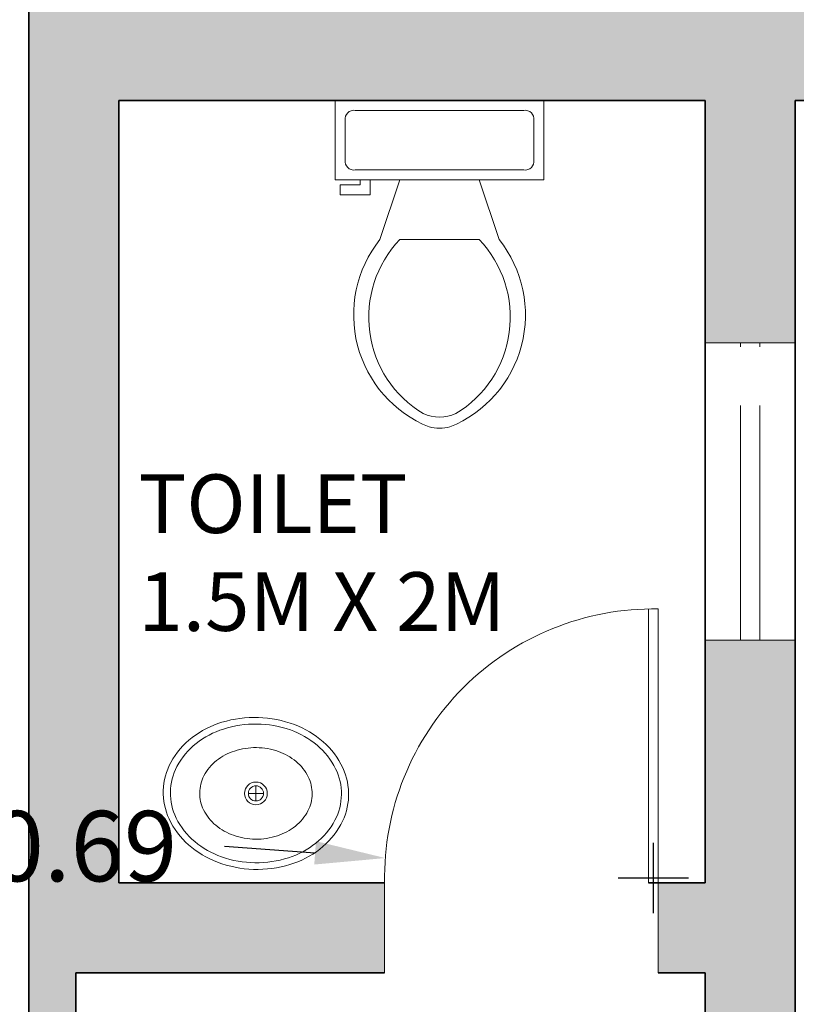
# Model space of a CAD drawing. Units: metres. Extents: x 4298.5 to 4325.2, y 2075 to 2095.8.
# Tile 28 of 35: x 4318.3 to 4320.3, y 2082.2 to 2084.8. Entities that reach past the tile are written whole.
import ezdxf

# ---------------------------------------------------------------- set-up
doc = ezdxf.new("R2010")
doc.units = ezdxf.units.M
doc.linetypes.add('ACAD_ISO02W100', pattern=[15, 12, -3])
for name, color, linetype, lineweight in [('A-ANNO-DIMS', 2, 'Continuous', 18), ('A-AREA-IDEN', 7, 'Continuous', 18), ('A-DOOR', 3, 'Continuous', 18), ('A-FLOR-FIXT', 15, 'Continuous', 18), ('A-GLAZ', 4, 'Continuous', 18), ('A-GLAZ-OVHD', 4, 'ACAD_ISO02W100', 13), ('A-WALL', 7, 'Continuous', 35), ('A-WALL-PATT', 252, 'Continuous', 13)]:
    doc.layers.add(name, color=color, linetype=linetype, lineweight=lineweight)
doc.styles.get("Standard").update_dxf_attribs({"font": 'arial.ttf'})
doc.dimstyles.get("Standard").update_dxf_attribs({"dimtxt": 0.18, "dimasz": 0.18, "dimexe": 0.18, "dimexo": 0.0625, "dimgap": 0.09, "dimtad": 0, "dimtih": 1, "dimtoh": 1, "dimdec": 4, "dimzin": 0, "dimdsep": 46, "dimtxsty": 'Standard', "dimcen": 0.09, "dimadec": 0, "dimazin": 0, "dimtfac": 1, "dimtdec": 4, "dimtofl": 0, "dimtmove": 0, "dimatfit": 3, "dimfxl": 1, "dimtolj": 1, "dimtzin": 0, "dimarcsym": 0})

# ---------------------------------------------------------------- blocks, each defined once
blk = doc.blocks.new('Toilet - top')
for p, q in [((9.5, -6), (9.5, -2)), ((-10, -8.5), (-8, -8.5)), ((-10, -9.5), (-10, -8.5)), ((-8, -8.5), (-8, -8)), ((-7, -8), (-7, -9.5)), ((-4, -8), (-6, -14)), ((4, -8), (6, -14)), ((-7, -9.5), (-10, -9.5)), ((4, -14), (-4, -14))]:
    blk.add_line(p, q)
blk.add_lwpolyline([(10.5, -8), (10.5, 0), (-10.5, 0), (-10.5, -8)], close=True)
for points in [[(8.5, -1), (-8.5, -1)], [(-9.5, -2), (-9.5, -6)], [(-8.5, -7), (8.5, -7)]]:
    blk.add_lwpolyline(points)
for centre, radius, start, end in [((-8.625, -1.875), 0.884, 81.8699, 188.1301), ((8.625, -1.875), 0.884, 351.8699, 98.1301), ((-8.625, -6.125), 0.884, 171.8699, 278.1301), ((8.625, -6.125), 0.884, 261.8699, 8.1301), ((3.52, -21.58), 12.169, 141.46911, 247.97143), ((4.2, -21.817), 11.329, 136.36773, 238.94682), ((-3.519, -21.58), 12.169, 292.02843, 38.53071), ((-4.2, -21.817), 11.329, 301.05301, 43.63209), ((0, -27.876), 4, 245.73182, 294.26817), ((0, -29), 4, 254.86053, 285.13947)]:
    blk.add_arc(centre, radius, start, end)
blk = doc.blocks.new('Sink - Oval top')
for p, q in [((-1, 0), (1, 0)), ((0, 1), (0, -1))]:
    blk.add_line(p, q)
for points in [[(-12.23, 0.39, 0.117634), (-11.46, -3.36, 0.104469), (-8.88, -6.8, 0.090016), (-5.08, -9.07, 0.08192), (-0.32, -10.02, 0.08192), (4.49, -9.38, 0.090016), (8.42, -7.36, 0.104469), (11.22, -4.09, 0.117634), (12.23, -0.39, 0.117634), (11.46, 3.36, 0.104469), (8.88, 6.8, 0.090016), (5.08, 9.07, 0.08192), (0.32, 10.02, 0.08192), (-4.49, 9.38, 0.090016), (-8.42, 7.36, 0.104469), (-11.22, 4.09, 0.117634)], [(-11.29, 0.16, 0.118622), (-10.52, -3.25, 0.104678), (-8.07, -6.36, 0.089562), (-4.54, -8.37, 0.081185), (-0.13, -9.15, 0.081185), (4.3, -8.49, 0.089562), (7.89, -6.58, 0.104678), (10.42, -3.55, 0.118622), (11.29, -0.16, 0.118622), (10.52, 3.25, 0.104678), (8.07, 6.36, 0.089562), (4.54, 8.37, 0.081185), (0.13, 9.15, 0.081185), (-4.3, 8.49, 0.089562), (-7.89, 6.58, 0.104678), (-10.42, 3.55, 0.118622)], [(-7.42, 0.08, 0.118283), (-6.91, -2.17, 0.104607), (-5.29, -4.21, 0.089718), (-2.97, -5.53, 0.081436), (-0.07, -6.04, 0.081436), (2.84, -5.59, 0.089718), (5.2, -4.33, 0.104607), (6.86, -2.32, 0.118283), (7.42, -0.08, 0.118283), (6.91, 2.17, 0.104607), (5.29, 4.21, 0.089718), (2.97, 5.53, 0.081436), (0.07, 6.04, 0.081436), (-2.84, 5.59, 0.089718), (-5.2, 4.33, 0.104607), (-6.86, 2.32, 0.118283)]]:
    blk.add_lwpolyline(points, format="xyb", close=True)
for radius in [1.5, 1]:
    blk.add_circle((0, 0), radius)
blk = doc.blocks.new('WIN-760-GLASS-HIGH')
at = {"ltscale": 0.05}
for p, q in [((0, 0.76), (0, 0)), ((0.05, 0.76), (0.05, 0))]:
    blk.add_line(p, q, dxfattribs=at)
blk = doc.blocks.new('DOOR-700-LEAF')
for p, q in [((0.675, 0), (0.675, 0.7)), ((0.7, 0), (0.7, 0.7))]:
    blk.add_line(p, q)
blk.add_arc((0.6875, 0.0125), 0.6876, 88.9584, 181.0416)
blk = doc.blocks.new('*D47')
at = {"layer": 'A-ANNO-DIMS', "color": 0, "lineweight": -2, "transparency": 16777216}
for p, q in [((4300.4306, 2084.4956), (4300.4306, 2074.9896)), ((4322.8106, 2084.4956), (4322.8106, 2074.9896)), ((4300.6106, 2075.1696), (4311.2252, 2075.1696)), ((4322.6306, 2075.1696), (4312.016, 2075.1696))]:
    blk.add_line(p, q, dxfattribs=at)
at = {"layer": 'A-ANNO-DIMS', "color": 0, "transparency": 16777216}
for points in [[(4300.6106, 2075.1996), (4300.6106, 2075.1396), (4300.4306, 2075.1696)], [(4322.6306, 2075.1996), (4322.6306, 2075.1396), (4322.8106, 2075.1696)]]:
    blk.add_solid(points, dxfattribs=at)
at = {"layer": 'Defpoints', "color": 0, "transparency": 16777216}
for p in [(4300.4306, 2084.5581), (4322.8106, 2084.5581), (4322.8106, 2075.1696)]:
    blk.add_point(p, dxfattribs=at)
at = {"layer": 'A-ANNO-DIMS', "color": 0, "transparency": 16777216, "insert": (4311.6206, 2075.1696), "char_height": 0.18, "attachment_point": 5}
blk.add_mtext('\\A1;22.38', dxfattribs=at)
blk = doc.blocks.new('*D48')
at = {"layer": 'A-ANNO-DIMS', "color": 0, "lineweight": -2, "transparency": 16777216}
for p, q in [((4310.1831, 2094.4781), (4324.7671, 2094.4781)), ((4324.5871, 2094.2981), (4324.5871, 2085.585)), ((4324.5871, 2076.5081), (4324.5871, 2085.2212)), ((4316.8731, 2076.3281), (4324.7671, 2076.3281))]:
    blk.add_line(p, q, dxfattribs=at)
at = {"layer": 'A-ANNO-DIMS', "color": 0, "transparency": 16777216}
for points in [[(4324.5571, 2094.2981), (4324.6171, 2094.2981), (4324.5871, 2094.4781)], [(4324.5571, 2076.5081), (4324.6171, 2076.5081), (4324.5871, 2076.3281)]]:
    blk.add_solid(points, dxfattribs=at)
at = {"layer": 'Defpoints', "color": 0, "transparency": 16777216}
for p in [(4310.1206, 2094.4781), (4316.8106, 2076.3281), (4324.5871, 2076.3281)]:
    blk.add_point(p, dxfattribs=at)
at = {"layer": 'A-ANNO-DIMS', "color": 0, "transparency": 16777216, "insert": (4324.5871, 2085.4031), "char_height": 0.18, "attachment_point": 5}
blk.add_mtext('\\A1;18.15', dxfattribs=at)
blk = doc.blocks.new('*D61')
at = {"layer": 'A-ANNO-DIMS', "color": 0, "lineweight": -2, "transparency": 16777216}
for p, q in [((4317.324045, 2083.575187), (4317.324045, 2095.816556)), ((4318.350577, 2084.620556), (4318.350577, 2095.816556)), ((4317.144045, 2095.636556), (4316.964045, 2095.636556)), ((4318.530577, 2095.636556), (4318.710577, 2095.636556))]:
    blk.add_line(p, q, dxfattribs=at)
at = {"layer": 'A-ANNO-DIMS', "color": 0, "transparency": 16777216}
for points in [[(4317.144045, 2095.666556), (4317.144045, 2095.606556), (4317.324045, 2095.636556)], [(4318.530577, 2095.666556), (4318.530577, 2095.606556), (4318.350577, 2095.636556)]]:
    blk.add_solid(points, dxfattribs=at)
at = {"layer": 'Defpoints', "color": 0, "transparency": 16777216}
for p in [(4318.350577, 2095.636556), (4318.350577, 2084.558056), (4317.324045, 2083.512687)]:
    blk.add_point(p, dxfattribs=at)
at = {"layer": 'A-ANNO-DIMS', "color": 0, "transparency": 16777216, "insert": (4317.837311, 2095.636556), "char_height": 0.18, "attachment_point": 5}
blk.add_mtext('\\A1;1.03', dxfattribs=at)
blk = doc.blocks.new('*D81')
at = {"layer": 'A-ANNO-DIMS', "color": 0, "lineweight": -2, "transparency": 16777216}
for p, q in [((4319.9481, 2082.4806), (4319.9481, 2082.6606)), ((4318.8509, 2082.6518), (4319.0828, 2082.6346)), ((4319.8581, 2082.5706), (4320.0381, 2082.5706))]:
    blk.add_line(p, q, dxfattribs=at)
at = {"layer": 'A-ANNO-DIMS', "color": 0, "transparency": 16777216}
blk.add_solid([(4319.085, 2082.6645), (4319.0806, 2082.6047), (4319.2623, 2082.6213)], dxfattribs=at)
at = {"layer": 'Defpoints', "color": 0, "transparency": 16777216}
for p in [(4319.2623, 2082.6213), (4319.9481, 2082.5706)]:
    blk.add_point(p, dxfattribs=at)
at = {"layer": 'A-ANNO-DIMS', "color": 0, "transparency": 16777216, "insert": (4318.2474, 2082.6518), "char_height": 0.18, "attachment_point": 5}
blk.add_mtext('\\A1;5X R0.69', dxfattribs=at)

msp = doc.modelspace()

# ---------------------------------------------------------------- hatches: boundary and pattern name
at = {"layer": 'A-WALL-PATT'}
h = msp.add_hatch(color=256, dxfattribs=at)
h.dxf.hatch_style = 1
h.paths.add_polyline_path([(4308.7606, 2094.4781), (4308.1606, 2094.4781), (4307.4606, 2094.4781), (4307.4606, 2094.2481), (4308.2706, 2094.2481), (4308.2706, 2094.1281), (4308.3906, 2094.1281), (4308.3906, 2094.2481), (4308.7606, 2094.2481)])
h.paths.add_polyline_path([(4310.1206, 2094.4781), (4309.5206, 2094.4781), (4309.5206, 2094.2481), (4309.8906, 2094.2481), (4309.8906, 2092.2481), (4308.3906, 2092.2481), (4308.3906, 2093.4281), (4308.2706, 2093.4281), (4308.2706, 2092.0181), (4309.8906, 2092.0181), (4309.8906, 2087.0181), (4309.7706, 2087.0181), (4309.7706, 2086.7881), (4309.8906, 2086.7881), (4311.9406, 2086.7881), (4311.9406, 2087.0181), (4310.1206, 2087.0181), (4310.1206, 2089.0181), (4310.2406, 2089.0181), (4310.2406, 2089.1381), (4310.1206, 2089.1381), (4310.1206, 2092.0181), (4310.3078, 2092.0181), (4310.3078, 2092.2481), (4310.1206, 2092.2481)])
h.paths.add_polyline_path([(4311.7406, 2092.2481), (4311.0678, 2092.2481), (4311.0678, 2092.0181), (4311.7406, 2092.0181)], flags=17)
h.paths.add_polyline_path([(4313.1733, 2092.2481), (4312.5006, 2092.2481), (4312.5006, 2092.0181), (4313.1733, 2092.0181)])
h.paths.add_polyline_path([(4314.5378, 2092.2481), (4314.1206, 2092.2481), (4313.9333, 2092.2481), (4313.9333, 2092.0181), (4314.1206, 2092.0181), (4314.1206, 2087.0181), (4314.0006, 2087.0181), (4314.0006, 2086.7881), (4314.1206, 2086.7881), (4315.5718, 2086.7881), (4315.5718, 2087.0181), (4314.3506, 2087.0181), (4314.3506, 2092.0181), (4314.5378, 2092.0181)])
h.paths.add_polyline_path([(4315.9706, 2092.2481), (4315.2978, 2092.2481), (4315.2978, 2092.0181), (4315.9706, 2092.0181)])
h.paths.add_polyline_path([(4317.4033, 2092.2481), (4316.7306, 2092.2481), (4316.7306, 2092.0181), (4317.4033, 2092.0181)])
h.paths.add_polyline_path([(4318.9506, 2092.2481), (4318.3506, 2092.2481), (4318.1633, 2092.2481), (4318.1633, 2092.0181), (4318.3506, 2092.0181), (4318.3506, 2091.8981), (4318.5806, 2091.8981), (4318.5806, 2092.0181), (4318.9506, 2092.0181)])
h.paths.add_polyline_path([(4321.0106, 2092.2481), (4319.7106, 2092.2481), (4319.7106, 2092.0181), (4320.0806, 2092.0181), (4320.0806, 2090.0181), (4318.5806, 2090.0181), (4318.5806, 2091.1981), (4318.3506, 2091.1981), (4318.3506, 2090.0181), (4318.3506, 2087.0181), (4318.2306, 2087.0181), (4318.2306, 2086.7881), (4318.3506, 2086.7881), (4318.3506, 2086.3081), (4318.5806, 2086.3081), (4318.5806, 2089.7881), (4321.7806, 2089.7881), (4321.7806, 2090.0181), (4320.2006, 2090.0181), (4320.2006, 2092.0181), (4321.0106, 2092.0181)])
h.paths.add_polyline_path([(4322.8106, 2092.2481), (4321.7706, 2092.2481), (4321.7706, 2092.0181), (4322.5806, 2092.0181), (4322.5806, 2091.2831), (4322.8106, 2091.2831)])
h.paths.add_polyline_path([(4322.8106, 2090.5231), (4322.5806, 2090.5231), (4322.5806, 2089.7881), (4322.5806, 2089.5254), (4322.8106, 2089.5254), (4322.8106, 2090.0181)])
h.paths.add_polyline_path([(4322.8106, 2088.7654), (4322.5806, 2088.7654), (4322.5806, 2087.6681), (4322.8106, 2087.6681)])
h.paths.add_polyline_path([(4322.8106, 2086.9081), (4322.5806, 2086.9081), (4322.5806, 2085.8107), (4322.8106, 2085.8107)])
h.paths.add_polyline_path([(4322.8106, 2085.0507), (4322.5806, 2085.0507), (4322.5806, 2084.7881), (4318.5806, 2084.7881), (4318.5806, 2085.0581), (4318.5806, 2085.4081), (4318.3506, 2085.4081), (4318.3506, 2084.5581), (4318.3506, 2080.8581), (4318.4706, 2080.8581), (4318.4706, 2082.3281), (4319.2606, 2082.3281), (4319.2606, 2082.5581), (4318.5806, 2082.5581), (4318.5806, 2084.5581), (4320.0806, 2084.5581), (4320.0806, 2083.9381), (4320.3106, 2083.9381), (4320.3106, 2084.5581), (4322.8106, 2084.5581)])
h.paths.add_polyline_path([(4320.3106, 2083.1781), (4320.0806, 2083.1781), (4320.0806, 2082.5581), (4319.9606, 2082.5581), (4319.9606, 2082.3281), (4320.0806, 2082.3281), (4320.0806, 2081.5731), (4320.3106, 2081.5731)], flags=17)
h.paths.add_polyline_path([(4320.3106, 2080.8131), (4320.0806, 2080.8131), (4320.0806, 2080.0581), (4318.4286, 2080.0581), (4318.4286, 2079.8281), (4320.3106, 2079.8281)])
h.paths.add_polyline_path([(4317.3506, 2085.2881), (4316.5718, 2085.2881), (4316.5718, 2085.0581), (4317.3506, 2085.0581)])
h.paths.add_polyline_path([(4315.5718, 2085.2881), (4314.8434, 2085.2881), (4314.8434, 2085.0581), (4315.5718, 2085.0581)])
h.paths.add_polyline_path([(4313.8434, 2085.2881), (4312.9406, 2085.2881), (4312.9406, 2085.0581), (4313.8434, 2085.0581)])
h.paths.add_polyline_path([(4311.9406, 2085.2881), (4311.4406, 2085.2881), (4311.4406, 2085.0581), (4311.9406, 2085.0581)])
h.paths.add_polyline_path([(4317.3306, 2087.0181), (4316.5718, 2087.0181), (4316.5718, 2086.7881), (4317.3306, 2086.7881)])
h.paths.add_polyline_path([(4313.1006, 2089.1381), (4311.1406, 2089.1381), (4311.1406, 2089.0181), (4312.9806, 2089.0181), (4312.9806, 2087.0181), (4312.9406, 2087.0181), (4312.9406, 2086.7881), (4313.1006, 2086.7881), (4313.1006, 2087.0181)])
h.paths.add_polyline_path([(4307.5515, 2087.0181), (4305.8906, 2087.0181), (4305.8906, 2092.2481), (4305.8906, 2094.2481), (4306.7006, 2094.2481), (4306.7006, 2094.4781), (4305.6606, 2094.4781), (4305.6606, 2092.2481), (4305.2906, 2092.2481), (4305.2906, 2092.0181), (4305.6606, 2092.0181), (4305.6606, 2090.0181), (4304.1606, 2090.0181), (4304.1606, 2091.1981), (4304.0406, 2091.1981), (4304.0406, 2089.9081), (4301.5606, 2089.9081), (4301.5606, 2089.7881), (4304.0406, 2089.7881), (4305.6606, 2089.7881), (4305.6606, 2086.6381), (4305.8906, 2086.6381), (4305.8906, 2086.7881), (4307.5515, 2086.7881)])
h.paths.add_polyline_path([(4307.5515, 2085.2881), (4305.8906, 2085.2881), (4305.8906, 2085.4381), (4305.6606, 2085.4381), (4305.6606, 2084.7881), (4305.2906, 2084.7881), (4305.2906, 2084.5581), (4305.6606, 2084.5581), (4305.6606, 2084.02), (4305.8906, 2084.02), (4305.8906, 2084.5581), (4305.8906, 2085.0581), (4307.5515, 2085.0581)])
h.paths.add_polyline_path([(4310.2406, 2085.2881), (4308.5515, 2085.2881), (4308.5515, 2085.0581), (4310.2406, 2085.0581)])
h.paths.add_polyline_path([(4317.4286, 2080.0581), (4316.5718, 2080.0581), (4316.5718, 2079.8281), (4317.4286, 2079.8281)])
h.paths.add_polyline_path([(4315.5718, 2080.0581), (4314.8434, 2080.0581), (4314.8434, 2079.8281), (4315.5718, 2079.8281)])
h.paths.add_polyline_path([(4313.8434, 2080.0581), (4312.9406, 2080.0581), (4312.9406, 2079.8281), (4313.8434, 2079.8281)])
h.paths.add_polyline_path([(4311.9406, 2080.0581), (4311.4406, 2080.0581), (4311.4406, 2079.8281), (4311.9406, 2079.8281)])
h.paths.add_polyline_path([(4310.2406, 2080.0581), (4310.1206, 2080.0581), (4310.1206, 2084.0381), (4309.8906, 2084.0381), (4309.8906, 2080.0581), (4309.1606, 2080.0581), (4309.1606, 2079.8281), (4310.2406, 2079.8281)])
h.paths.add_polyline_path([(4308.1606, 2080.0581), (4307.5106, 2080.0581), (4307.5106, 2080.1781), (4307.3906, 2080.1781), (4307.3906, 2080.0581), (4305.8906, 2080.0581), (4305.8906, 2080.567), (4305.6606, 2080.567), (4305.6606, 2079.8281), (4308.1606, 2079.8281)])
h.paths.add_polyline_path([(4307.5106, 2081.9381), (4309.0906, 2081.9381), (4309.0906, 2082.0581), (4305.8906, 2082.0581), (4305.8906, 2083.26), (4305.6606, 2083.26), (4305.6606, 2081.327), (4305.8906, 2081.327), (4305.8906, 2081.9381), (4307.3906, 2081.9381), (4307.3906, 2080.8781), (4307.5106, 2080.8781)])
h.paths.add_polyline_path([(4304.5306, 2084.7881), (4302.7306, 2084.7881), (4302.7306, 2084.5581), (4304.5306, 2084.5581)])
h.paths.add_polyline_path([(4301.9706, 2084.7881), (4300.6606, 2084.7881), (4300.6606, 2085.0249), (4300.4306, 2085.0249), (4300.4306, 2084.5581), (4301.9706, 2084.5581)])
h.paths.add_polyline_path([(4300.6606, 2086.8843), (4300.4306, 2086.8843), (4300.4306, 2085.7849), (4300.6606, 2085.7849)])
h.paths.add_polyline_path([(4300.6606, 2089.1618), (4300.4306, 2089.1618), (4300.4306, 2087.6443), (4300.6606, 2087.6443)])
h.paths.add_polyline_path([(4300.6606, 2091.0212), (4300.4306, 2091.0212), (4300.4306, 2089.9218), (4300.6606, 2089.9218)])
h.paths.add_polyline_path([(4300.6606, 2092.0181), (4301.9706, 2092.0181), (4301.9706, 2092.2481), (4300.4306, 2092.2481), (4300.4306, 2091.7812), (4300.6606, 2091.7812)])
h.paths.add_polyline_path([(4304.5306, 2092.2481), (4302.7306, 2092.2481), (4302.7306, 2092.0181), (4304.0406, 2092.0181), (4304.0406, 2091.8981), (4304.1606, 2091.8981), (4304.1606, 2092.0181), (4304.5306, 2092.0181)], flags=17)

# ---------------------------------------------------------------- linework, layer by layer
at = {"layer": 'A-DOOR'}
for p, q in [((4319.2606, 2082.5581), (4319.2606, 2082.3281)), ((4319.9606, 2082.5581), (4319.9606, 2082.3281))]:
    msp.add_line(p, q, dxfattribs=at)
at = {"layer": 'A-GLAZ'}
for p, q in [((4320.0806, 2083.9381), (4320.3106, 2083.9381)), ((4320.0806, 2083.1781), (4320.3106, 2083.1781))]:
    msp.add_line(p, q, dxfattribs=at)
at = {"layer": 'A-WALL'}
for p, q in [((4318.3506, 2084.5581), (4318.3506, 2085.4081)), ((4318.3506, 2085.0581), (4318.3506, 2080.8581)), ((4318.5806, 2084.5581), (4318.5806, 2082.5581)), ((4320.0806, 2084.5581), (4318.5806, 2084.5581)), ((4320.0806, 2084.5581), (4320.0806, 2082.5581)), ((4322.8106, 2084.5581), (4320.3106, 2084.5581)), ((4320.3106, 2084.5581), (4320.3106, 2079.8281)), ((4319.2606, 2082.5581), (4318.5806, 2082.5581)), ((4320.0806, 2082.5581), (4319.9356, 2082.5581)), ((4318.4706, 2082.3281), (4318.4706, 2080.8581)), ((4319.2606, 2082.3281), (4318.4706, 2082.3281)), ((4320.0806, 2082.3281), (4319.9606, 2082.3281)), ((4320.0806, 2082.3281), (4320.0806, 2080.0581))]:
    msp.add_line(p, q, dxfattribs=at)

# ---------------------------------------------------------------- block references
at = {"layer": 'A-DOOR'}
msp.add_blockref('DOOR-700-LEAF', (4319.2605, 2082.5581), dxfattribs=at)
at = {"layer": 'A-FLOR-FIXT'}
for name, p, xscale, yscale, zscale in [('Toilet - top', (4319.401, 2084.5581), 0.0254, 0.0254, 0.0254), ('Sink - Oval top', (4318.9314, 2082.7866), 0.0193818050953029, 0.0193818050953029, 0.0193818050953029)]:
    msp.add_blockref(name, p, dxfattribs=dict(at, xscale=xscale, yscale=yscale, zscale=zscale))
at = {"layer": 'A-GLAZ-OVHD', "rotation": 180}
msp.add_blockref('WIN-760-GLASS-HIGH', (4320.2206, 2083.9381), dxfattribs=at)

# ---------------------------------------------------------------- texts
at = {"layer": 'A-AREA-IDEN', "insert": (4318.6308, 2083.6021), "char_height": 0.15, "attachment_point": 1}
msp.add_mtext_dynamic_manual_height_columns('TOILET\\P1.5M X 2M', width=2.22034, gutter_width=12.5, heights=[0], dxfattribs=at)

# ---------------------------------------------------------------- dimensions: what is measured, and where the dimension line sits
at = {"layer": 'A-ANNO-DIMS'}
for base, p1, p2, picture, middle in [((4318.3506, 2095.6366), (4317.324, 2083.5127), (4318.3506, 2084.5581), '*D61', (4317.8373, 2095.6366)), ((4322.8106, 2075.1696), (4300.4306, 2084.5581), (4322.8106, 2084.5581), '*D47', (4311.6206, 2075.1696))]:
    dim = msp.add_linear_dim(base=base, p1=p1, p2=p2, dimstyle='Standard', override={"dimdec": 2, "dimlfac": 1, "dimrnd": 0, "dimzin": 0, "dimdsep": 46, "dimlunit": 2}, dxfattribs=at)
    dim.commit()
    dim.dimension.update_dxf_attribs({"geometry": picture, "text_midpoint": middle})
dim = msp.add_linear_dim(base=(4324.5871, 2076.3281), p1=(4310.1206, 2094.4781), p2=(4316.8106, 2076.3281), angle=90, dimstyle='Standard', override={"dimdec": 2, "dimlfac": 1, "dimrnd": 0, "dimzin": 0, "dimdsep": 46, "dimlunit": 2}, dxfattribs=at)
dim.commit()
dim.dimension.update_dxf_attribs({"geometry": '*D48', "text_midpoint": (4324.5871, 2085.4031)})
dim = msp.add_radius_dim(center=(4319.9481, 2082.5706), mpoint=(4319.2623, 2082.6213), text='5X <>', dimstyle='Standard', override={"dimdec": 2, "dimlfac": 1, "dimrnd": 0, "dimzin": 0, "dimdsep": 46, "dimlunit": 2}, dxfattribs=at)
dim.commit()
dim.dimension.update_dxf_attribs({"geometry": '*D81', "text_midpoint": (4318.8509, 2082.6518), "dimtype": 164})

doc.saveas('drawing.dxf')
